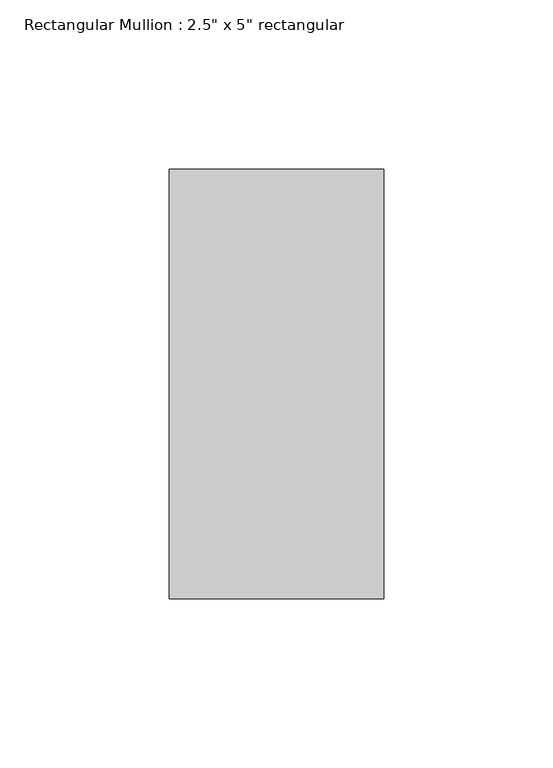
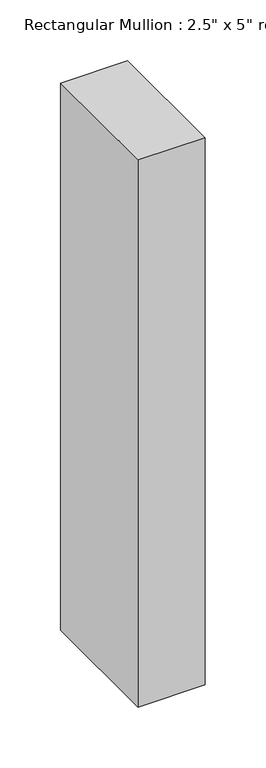
"""IFC4 building model written with IfcOpenShell, lengths in millimetres: member geometry."""

from ifc_helpers import new_model, si_unit, frame, origin, place, context, project, spatial, polyline, outline, extrude, source, transform, mapped, element, save


def member_544ec0ca(model_context):
    return source(origin(), model_context, "Body", "SweptSolid", [
        extrude(outline(polyline([(0.0, 63.5), (0.0, -63.5), (-63.5, -63.5), (-63.5, 63.5), (0.0, 63.5)])), frame((0.0, 0.0, -548.7736842), z_axis=(0.0, 0.0, 1.0), x_axis=(1.0, 0.0, 0.0)), (0.0, 0.0, 1.0), 548.7736842),
    ])


if __name__ == "__main__":
    model = new_model("IFC4")
    model_context = context("Model", 3, world=origin())
    ifc_project = project(units=[si_unit("LENGTHUNIT", "METRE", prefix="MILLI")], contexts=[model_context])
    site = spatial("IfcSite", under=ifc_project)
    building = spatial("IfcBuilding", under=site)
    placement = place(None, origin())
    member_shape = member_544ec0ca(model_context)
    element("IfcMember", 1, ObjectType="Rectangular Mullion : 2.5\" x 5\" rectangular", at=placement, inside=building, context=model_context, shape_type="MappedRepresentation", body=[
        mapped(member_shape, transform((0.0, 0.0, 0.0), x_axis=(1.0, 0.0, 0.0), y_axis=(0.0, 1.0, 0.0), z_axis=(0.0, 0.0, 1.0))),
    ])
    save(model, "model.ifc")

# Revit data of these elements
# Type "Rectangular Mullion : 2.5\" x 5\" rectangular"
#   built-in parameter 1007304 = 0.416667 (stored number, unit not read)
#   built-in parameter 1007301 = 0.104167 (stored number, unit not read)
#   built-in parameter 1007300 = 0.104167 (stored number, unit not read)
# Element 1 (IfcMember, "Rectangular Mullion : 2.5\" x 5\" rectangular")
#   Materials on its faces: "Aluminum"
# Materials
#   "Aluminum": class "Metal", colour RGB 247 247 247, transparency 0, Description = "Aluminum 6061", Cost = 0
